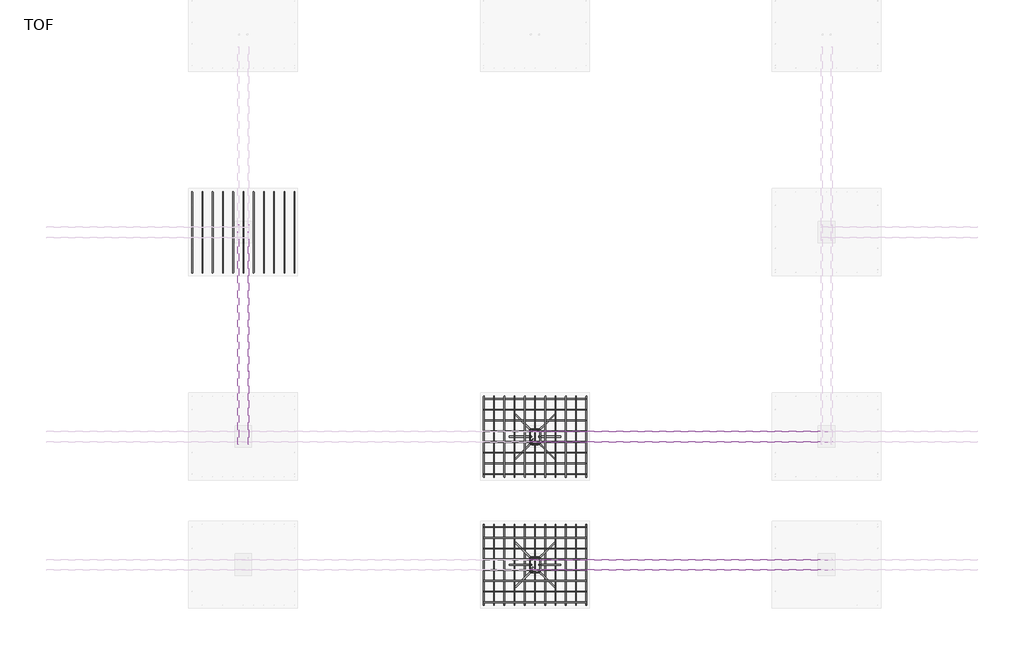
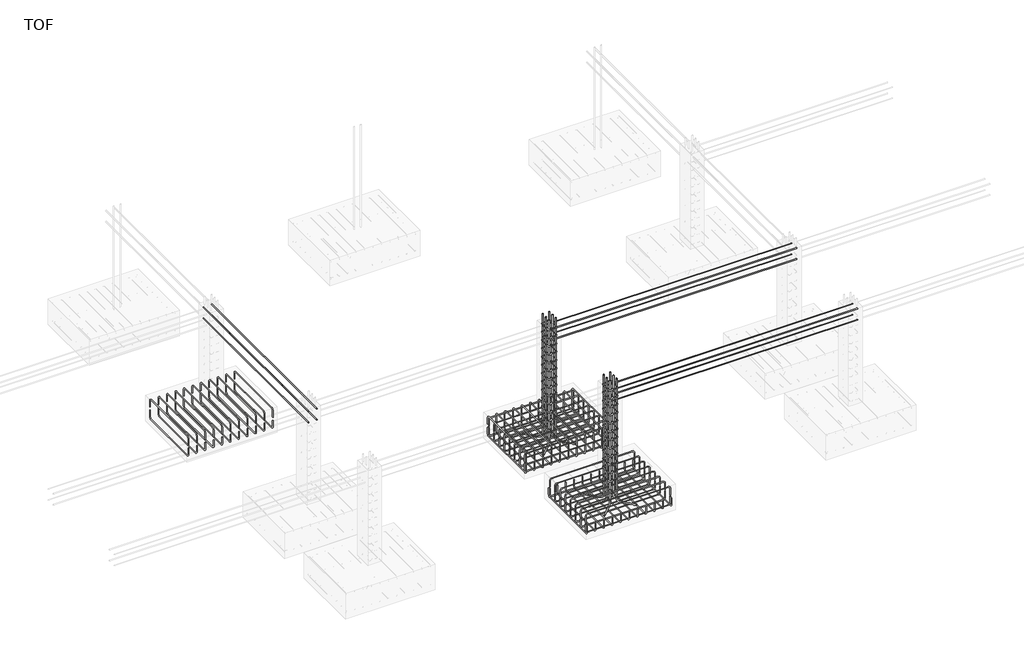
# One storey, part 5 of 10: 35 reinforcing bars.
"""IFC4 building model written with IfcOpenShell, lengths in millimetres."""

from ifc_helpers import new_model, si_unit, point, frame, origin, place, context, project, spatial, polyline, circle_curve, trimmed, segment, composite_curve, source, transform, mapped, element, save
from ifc_brep_helpers import swept_disk

model = new_model("IFC4")

# Units and contexts
model_context = context("Model", 3, world=origin())
ifc_project = project(units=[si_unit("LENGTHUNIT", "METRE", prefix="MILLI")], contexts=[model_context])

# Site, building, storey
site = spatial("IfcSite", under=ifc_project)
building = spatial("IfcBuilding", under=site)
storey = spatial("IfcBuildingStorey", under=building, Name="TOF", Elevation=-1828.8)

# Reinforcing bars
placement = place(None, origin())
reinforcing_bar_shape = source(origin(), model_context, "Body", "SolidModel", [
    swept_disk(composite_curve([segment(polyline([(6330.2782143, -15649.6267376, -2077.5233378), (6330.2782143, -15649.6267376, -2187.5233378)]), True, "CONTINUOUS"), segment(trimmed(circle_curve(frame((6330.2782143, -15614.6267376, -2187.5233378), z_axis=(1.0, 0.0, 0.0), x_axis=(0.0, -35.0, 0.0)), 35.0), [point((6330.2782143, -15649.6267376, -2187.5233378))], [point((6330.2782143, -15614.6267376, -2222.5233378))], True, "CARTESIAN"), True, "CONTINUOUS"), segment(polyline([(6330.2782143, -15614.6267376, -2222.5233378), (6330.2782143, -14574.6267376, -2222.5233378)]), True, "CONTINUOUS"), segment(trimmed(circle_curve(frame((6330.2782143, -14574.6267376, -2187.5233378), z_axis=(1.0, 0.0, 0.0), x_axis=(0.0, 0.0, -35.0)), 35.0), [point((6330.2782143, -14574.6267376, -2222.5233378))], [point((6330.2782143, -14539.6267376, -2187.5233378))], True, "CARTESIAN"), True, "CONTINUOUS"), segment(polyline([(6330.2782143, -14539.6267376, -2187.5233378), (6330.2782143, -14539.6267376, -2077.5233378)]), True, "CONTINUOUS")], self_intersect=False), 5.0),
])
element("IfcReinforcingBar", 1, at=placement, inside=storey, context=model_context, shape_type="MappedRepresentation", body=[
    mapped(reinforcing_bar_shape, transform((0.0, 0.0, 0.0), x_axis=(1.0, 0.0, 0.0), y_axis=(0.0, 1.0, 0.0), z_axis=(0.0, 0.0, 1.0))),
    mapped(reinforcing_bar_shape, transform((-141.0, 0.0, 0.0), x_axis=(1.0, 0.0, 0.0), y_axis=(0.0, 1.0, 0.0), z_axis=(0.0, 0.0, 1.0))),
    mapped(reinforcing_bar_shape, transform((-282.0, 0.0, 0.0), x_axis=(1.0, 0.0, 0.0), y_axis=(0.0, 1.0, 0.0), z_axis=(0.0, 0.0, 1.0))),
    mapped(reinforcing_bar_shape, transform((-423.0, 0.0, 0.0), x_axis=(1.0, 0.0, 0.0), y_axis=(0.0, 1.0, 0.0), z_axis=(0.0, 0.0, 1.0))),
    mapped(reinforcing_bar_shape, transform((-564.0, 0.0, 0.0), x_axis=(1.0, 0.0, 0.0), y_axis=(0.0, 1.0, 0.0), z_axis=(0.0, 0.0, 1.0))),
    mapped(reinforcing_bar_shape, transform((-705.0, 0.0, 0.0), x_axis=(1.0, 0.0, 0.0), y_axis=(0.0, 1.0, 0.0), z_axis=(0.0, 0.0, 1.0))),
    mapped(reinforcing_bar_shape, transform((-846.0, 0.0, 0.0), x_axis=(1.0, 0.0, 0.0), y_axis=(0.0, 1.0, 0.0), z_axis=(0.0, 0.0, 1.0))),
    mapped(reinforcing_bar_shape, transform((-987.0, 0.0, 0.0), x_axis=(1.0, 0.0, 0.0), y_axis=(0.0, 1.0, 0.0), z_axis=(0.0, 0.0, 1.0))),
    mapped(reinforcing_bar_shape, transform((-1128.0, 0.0, 0.0), x_axis=(1.0, 0.0, 0.0), y_axis=(0.0, 1.0, 0.0), z_axis=(0.0, 0.0, 1.0))),
    mapped(reinforcing_bar_shape, transform((-1269.0, 0.0, 0.0), x_axis=(1.0, 0.0, 0.0), y_axis=(0.0, 1.0, 0.0), z_axis=(0.0, 0.0, 1.0))),
    mapped(reinforcing_bar_shape, transform((-1410.0, 0.0, 0.0), x_axis=(1.0, 0.0, 0.0), y_axis=(0.0, 1.0, 0.0), z_axis=(0.0, 0.0, 1.0))),
])
reinforcing_bar_2_shape = source(origin(), model_context, "Body", "SolidModel", [
    swept_disk(composite_curve([segment(polyline([(6330.2782143, -14574.6861459, -2066.1776706), (6330.2782143, -14574.6861459, -2176.1776706)]), True, "CONTINUOUS"), segment(trimmed(circle_curve(frame((6295.2782143, -14574.6861459, -2176.1776706), z_axis=(0.0, 1.0, 0.0), x_axis=(35.0, 0.0, 0.0)), 35.0), [point((6330.2782143, -14574.6861459, -2176.1776706))], [point((6295.2782143, -14574.6861459, -2211.1776706))], True, "CARTESIAN"), True, "CONTINUOUS"), segment(polyline([(6295.2782143, -14574.6861459, -2211.1776706), (4955.2782143, -14574.6861459, -2211.1776706)]), True, "CONTINUOUS"), segment(trimmed(circle_curve(frame((4955.2782143, -14574.6861459, -2176.1776706), z_axis=(0.0, 1.0, 0.0), x_axis=(0.0, 0.0, -35.0)), 35.0), [point((4955.2782143, -14574.6861459, -2211.1776706))], [point((4920.2782143, -14574.6861459, -2176.1776706))], True, "CARTESIAN"), True, "CONTINUOUS"), segment(polyline([(4920.2782143, -14574.6861459, -2176.1776706), (4920.2782143, -14574.6861459, -2066.1776706)]), True, "CONTINUOUS")], self_intersect=False), 5.0),
])
element("IfcReinforcingBar", 2, at=placement, inside=storey, context=model_context, shape_type="MappedRepresentation", body=[
    mapped(reinforcing_bar_2_shape, transform((0.0, 0.0, 0.0), x_axis=(1.0, 0.0, 0.0), y_axis=(0.0, 1.0, 0.0), z_axis=(0.0, 0.0, 1.0))),
    mapped(reinforcing_bar_2_shape, transform((0.0, -148.0321606, 0.0), x_axis=(1.0, 0.0, 0.0), y_axis=(0.0, 1.0, 0.0), z_axis=(0.0, 0.0, 1.0))),
    mapped(reinforcing_bar_2_shape, transform((0.0, -296.0643211, 0.0), x_axis=(1.0, 0.0, 0.0), y_axis=(0.0, 1.0, 0.0), z_axis=(0.0, 0.0, 1.0))),
    mapped(reinforcing_bar_2_shape, transform((0.0, -444.0964817, 0.0), x_axis=(1.0, 0.0, 0.0), y_axis=(0.0, 1.0, 0.0), z_axis=(0.0, 0.0, 1.0))),
    mapped(reinforcing_bar_2_shape, transform((0.0, -592.1286423, 0.0), x_axis=(1.0, 0.0, 0.0), y_axis=(0.0, 1.0, 0.0), z_axis=(0.0, 0.0, 1.0))),
    mapped(reinforcing_bar_2_shape, transform((0.0, -740.1608029, 0.0), x_axis=(1.0, 0.0, 0.0), y_axis=(0.0, 1.0, 0.0), z_axis=(0.0, 0.0, 1.0))),
    mapped(reinforcing_bar_2_shape, transform((0.0, -888.1929634, 0.0), x_axis=(1.0, 0.0, 0.0), y_axis=(0.0, 1.0, 0.0), z_axis=(0.0, 0.0, 1.0))),
    mapped(reinforcing_bar_2_shape, transform((0.0, -1036.225124, 0.0), x_axis=(1.0, 0.0, 0.0), y_axis=(0.0, 1.0, 0.0), z_axis=(0.0, 0.0, 1.0))),
])
reinforcing_bar_3_shape = source(origin(), model_context, "Body", "SolidModel", [
    swept_disk(composite_curve([segment(polyline([(6330.2782143, -15610.9112699, -2039.256778), (6330.2782143, -15610.9112699, -1929.256778)]), True, "CONTINUOUS"), segment(trimmed(circle_curve(frame((6295.2782143, -15610.9112699, -1929.256778), z_axis=(0.0, -1.0, 0.0), x_axis=(35.0, 0.0, 0.0)), 35.0), [point((6330.2782143, -15610.9112699, -1929.256778))], [point((6295.2782143, -15610.9112699, -1894.256778))], True, "CARTESIAN"), True, "CONTINUOUS"), segment(polyline([(6295.2782143, -15610.9112699, -1894.256778), (4955.2782143, -15610.9112699, -1894.256778)]), True, "CONTINUOUS"), segment(trimmed(circle_curve(frame((4955.2782143, -15610.9112699, -1929.256778), z_axis=(0.0, -1.0, 0.0), x_axis=(0.0, 0.0, 35.0)), 35.0), [point((4955.2782143, -15610.9112699, -1894.256778))], [point((4920.2782143, -15610.9112699, -1929.256778))], True, "CARTESIAN"), True, "CONTINUOUS"), segment(polyline([(4920.2782143, -15610.9112699, -1929.256778), (4920.2782143, -15610.9112699, -2039.256778)]), True, "CONTINUOUS")], self_intersect=False), 5.0),
])
element("IfcReinforcingBar", 3, at=placement, inside=storey, context=model_context, shape_type="MappedRepresentation", body=[
    mapped(reinforcing_bar_3_shape, transform((0.0, 0.0, 0.0), x_axis=(1.0, 0.0, 0.0), y_axis=(0.0, 1.0, 0.0), z_axis=(0.0, 0.0, 1.0))),
    mapped(reinforcing_bar_3_shape, transform((0.0, 148.0321606, 0.0), x_axis=(1.0, 0.0, 0.0), y_axis=(0.0, 1.0, 0.0), z_axis=(0.0, 0.0, 1.0))),
    mapped(reinforcing_bar_3_shape, transform((0.0, 296.0643211, 0.0), x_axis=(1.0, 0.0, 0.0), y_axis=(0.0, 1.0, 0.0), z_axis=(0.0, 0.0, 1.0))),
    mapped(reinforcing_bar_3_shape, transform((0.0, 444.0964817, 0.0), x_axis=(1.0, 0.0, 0.0), y_axis=(0.0, 1.0, 0.0), z_axis=(0.0, 0.0, 1.0))),
    mapped(reinforcing_bar_3_shape, transform((0.0, 592.1286423, 0.0), x_axis=(1.0, 0.0, 0.0), y_axis=(0.0, 1.0, 0.0), z_axis=(0.0, 0.0, 1.0))),
    mapped(reinforcing_bar_3_shape, transform((0.0, 740.1608029, 0.0), x_axis=(1.0, 0.0, 0.0), y_axis=(0.0, 1.0, 0.0), z_axis=(0.0, 0.0, 1.0))),
    mapped(reinforcing_bar_3_shape, transform((0.0, 888.1929634, 0.0), x_axis=(1.0, 0.0, 0.0), y_axis=(0.0, 1.0, 0.0), z_axis=(0.0, 0.0, 1.0))),
    mapped(reinforcing_bar_3_shape, transform((0.0, 1036.225124, 0.0), x_axis=(1.0, 0.0, 0.0), y_axis=(0.0, 1.0, 0.0), z_axis=(0.0, 0.0, 1.0))),
])
reinforcing_bar_4_shape = source(origin(), model_context, "Body", "SolidModel", [
    swept_disk(composite_curve([segment(polyline([(6330.2782143, -12774.6267376, -2018.8), (6330.2782143, -12774.6267376, -1908.8)]), True, "CONTINUOUS"), segment(trimmed(circle_curve(frame((6330.2782143, -12809.6267376, -1908.8), z_axis=(1.0, 0.0, 0.0), x_axis=(0.0, 35.0, 0.0)), 35.0), [point((6330.2782143, -12774.6267376, -1908.8))], [point((6330.2782143, -12809.6267376, -1873.8))], True, "CARTESIAN"), True, "CONTINUOUS"), segment(polyline([(6330.2782143, -12809.6267376, -1873.8), (6330.2782143, -13849.6267376, -1873.8)]), True, "CONTINUOUS"), segment(trimmed(circle_curve(frame((6330.2782143, -13849.6267376, -1908.8), z_axis=(1.0, 0.0, 0.0), x_axis=(0.0, 0.0, 35.0)), 35.0), [point((6330.2782143, -13849.6267376, -1873.8))], [point((6330.2782143, -13884.6267376, -1908.8))], True, "CARTESIAN"), True, "CONTINUOUS"), segment(polyline([(6330.2782143, -13884.6267376, -1908.8), (6330.2782143, -13884.6267376, -2018.8)]), True, "CONTINUOUS")], self_intersect=False), 5.0),
])
element("IfcReinforcingBar", 4, at=placement, inside=storey, context=model_context, shape_type="MappedRepresentation", body=[
    mapped(reinforcing_bar_4_shape, transform((0.0, 0.0, 0.0), x_axis=(1.0, 0.0, 0.0), y_axis=(0.0, 1.0, 0.0), z_axis=(0.0, 0.0, 1.0))),
    mapped(reinforcing_bar_4_shape, transform((-141.0, 0.0, 0.0), x_axis=(1.0, 0.0, 0.0), y_axis=(0.0, 1.0, 0.0), z_axis=(0.0, 0.0, 1.0))),
    mapped(reinforcing_bar_4_shape, transform((-282.0, 0.0, 0.0), x_axis=(1.0, 0.0, 0.0), y_axis=(0.0, 1.0, 0.0), z_axis=(0.0, 0.0, 1.0))),
    mapped(reinforcing_bar_4_shape, transform((-423.0, 0.0, 0.0), x_axis=(1.0, 0.0, 0.0), y_axis=(0.0, 1.0, 0.0), z_axis=(0.0, 0.0, 1.0))),
    mapped(reinforcing_bar_4_shape, transform((-564.0, 0.0, 0.0), x_axis=(1.0, 0.0, 0.0), y_axis=(0.0, 1.0, 0.0), z_axis=(0.0, 0.0, 1.0))),
    mapped(reinforcing_bar_4_shape, transform((-705.0, 0.0, 0.0), x_axis=(1.0, 0.0, 0.0), y_axis=(0.0, 1.0, 0.0), z_axis=(0.0, 0.0, 1.0))),
    mapped(reinforcing_bar_4_shape, transform((-846.0, 0.0, 0.0), x_axis=(1.0, 0.0, 0.0), y_axis=(0.0, 1.0, 0.0), z_axis=(0.0, 0.0, 1.0))),
    mapped(reinforcing_bar_4_shape, transform((-987.0, 0.0, 0.0), x_axis=(1.0, 0.0, 0.0), y_axis=(0.0, 1.0, 0.0), z_axis=(0.0, 0.0, 1.0))),
    mapped(reinforcing_bar_4_shape, transform((-1128.0, 0.0, 0.0), x_axis=(1.0, 0.0, 0.0), y_axis=(0.0, 1.0, 0.0), z_axis=(0.0, 0.0, 1.0))),
    mapped(reinforcing_bar_4_shape, transform((-1269.0, 0.0, 0.0), x_axis=(1.0, 0.0, 0.0), y_axis=(0.0, 1.0, 0.0), z_axis=(0.0, 0.0, 1.0))),
    mapped(reinforcing_bar_4_shape, transform((-1410.0, 0.0, 0.0), x_axis=(1.0, 0.0, 0.0), y_axis=(0.0, 1.0, 0.0), z_axis=(0.0, 0.0, 1.0))),
])
reinforcing_bar_5_shape = source(origin(), model_context, "Body", "SolidModel", [
    swept_disk(composite_curve([segment(polyline([(6330.2782143, -13884.6267376, -2077.5233378), (6330.2782143, -13884.6267376, -2187.5233378)]), True, "CONTINUOUS"), segment(trimmed(circle_curve(frame((6330.2782143, -13849.6267376, -2187.5233378), z_axis=(1.0, 0.0, 0.0), x_axis=(0.0, -35.0, 0.0)), 35.0), [point((6330.2782143, -13884.6267376, -2187.5233378))], [point((6330.2782143, -13849.6267376, -2222.5233378))], True, "CARTESIAN"), True, "CONTINUOUS"), segment(polyline([(6330.2782143, -13849.6267376, -2222.5233378), (6330.2782143, -12809.6267376, -2222.5233378)]), True, "CONTINUOUS"), segment(trimmed(circle_curve(frame((6330.2782143, -12809.6267376, -2187.5233378), z_axis=(1.0, 0.0, 0.0), x_axis=(0.0, 0.0, -35.0)), 35.0), [point((6330.2782143, -12809.6267376, -2222.5233378))], [point((6330.2782143, -12774.6267376, -2187.5233378))], True, "CARTESIAN"), True, "CONTINUOUS"), segment(polyline([(6330.2782143, -12774.6267376, -2187.5233378), (6330.2782143, -12774.6267376, -2077.5233378)]), True, "CONTINUOUS")], self_intersect=False), 5.0),
])
element("IfcReinforcingBar", 5, at=placement, inside=storey, context=model_context, shape_type="MappedRepresentation", body=[
    mapped(reinforcing_bar_5_shape, transform((0.0, 0.0, 0.0), x_axis=(1.0, 0.0, 0.0), y_axis=(0.0, 1.0, 0.0), z_axis=(0.0, 0.0, 1.0))),
    mapped(reinforcing_bar_5_shape, transform((-141.0, 0.0, 0.0), x_axis=(1.0, 0.0, 0.0), y_axis=(0.0, 1.0, 0.0), z_axis=(0.0, 0.0, 1.0))),
    mapped(reinforcing_bar_5_shape, transform((-282.0, 0.0, 0.0), x_axis=(1.0, 0.0, 0.0), y_axis=(0.0, 1.0, 0.0), z_axis=(0.0, 0.0, 1.0))),
    mapped(reinforcing_bar_5_shape, transform((-423.0, 0.0, 0.0), x_axis=(1.0, 0.0, 0.0), y_axis=(0.0, 1.0, 0.0), z_axis=(0.0, 0.0, 1.0))),
    mapped(reinforcing_bar_5_shape, transform((-564.0, 0.0, 0.0), x_axis=(1.0, 0.0, 0.0), y_axis=(0.0, 1.0, 0.0), z_axis=(0.0, 0.0, 1.0))),
    mapped(reinforcing_bar_5_shape, transform((-705.0, 0.0, 0.0), x_axis=(1.0, 0.0, 0.0), y_axis=(0.0, 1.0, 0.0), z_axis=(0.0, 0.0, 1.0))),
    mapped(reinforcing_bar_5_shape, transform((-846.0, 0.0, 0.0), x_axis=(1.0, 0.0, 0.0), y_axis=(0.0, 1.0, 0.0), z_axis=(0.0, 0.0, 1.0))),
    mapped(reinforcing_bar_5_shape, transform((-987.0, 0.0, 0.0), x_axis=(1.0, 0.0, 0.0), y_axis=(0.0, 1.0, 0.0), z_axis=(0.0, 0.0, 1.0))),
    mapped(reinforcing_bar_5_shape, transform((-1128.0, 0.0, 0.0), x_axis=(1.0, 0.0, 0.0), y_axis=(0.0, 1.0, 0.0), z_axis=(0.0, 0.0, 1.0))),
    mapped(reinforcing_bar_5_shape, transform((-1269.0, 0.0, 0.0), x_axis=(1.0, 0.0, 0.0), y_axis=(0.0, 1.0, 0.0), z_axis=(0.0, 0.0, 1.0))),
    mapped(reinforcing_bar_5_shape, transform((-1410.0, 0.0, 0.0), x_axis=(1.0, 0.0, 0.0), y_axis=(0.0, 1.0, 0.0), z_axis=(0.0, 0.0, 1.0))),
])
reinforcing_bar_6_shape = source(origin(), model_context, "Body", "SolidModel", [
    swept_disk(composite_curve([segment(polyline([(6330.2782143, -12809.6861459, -2066.1776706), (6330.2782143, -12809.6861459, -2176.1776706)]), True, "CONTINUOUS"), segment(trimmed(circle_curve(frame((6295.2782143, -12809.6861459, -2176.1776706), z_axis=(0.0, 1.0, 0.0), x_axis=(35.0, 0.0, 0.0)), 35.0), [point((6330.2782143, -12809.6861459, -2176.1776706))], [point((6295.2782143, -12809.6861459, -2211.1776706))], True, "CARTESIAN"), True, "CONTINUOUS"), segment(polyline([(6295.2782143, -12809.6861459, -2211.1776706), (4955.2782143, -12809.6861459, -2211.1776706)]), True, "CONTINUOUS"), segment(trimmed(circle_curve(frame((4955.2782143, -12809.6861459, -2176.1776706), z_axis=(0.0, 1.0, 0.0), x_axis=(0.0, 0.0, -35.0)), 35.0), [point((4955.2782143, -12809.6861459, -2211.1776706))], [point((4920.2782143, -12809.6861459, -2176.1776706))], True, "CARTESIAN"), True, "CONTINUOUS"), segment(polyline([(4920.2782143, -12809.6861459, -2176.1776706), (4920.2782143, -12809.6861459, -2066.1776706)]), True, "CONTINUOUS")], self_intersect=False), 5.0),
])
element("IfcReinforcingBar", 6, at=placement, inside=storey, context=model_context, shape_type="MappedRepresentation", body=[
    mapped(reinforcing_bar_6_shape, transform((0.0, 0.0, 0.0), x_axis=(1.0, 0.0, 0.0), y_axis=(0.0, 1.0, 0.0), z_axis=(0.0, 0.0, 1.0))),
    mapped(reinforcing_bar_6_shape, transform((0.0, -148.0321606, 0.0), x_axis=(1.0, 0.0, 0.0), y_axis=(0.0, 1.0, 0.0), z_axis=(0.0, 0.0, 1.0))),
    mapped(reinforcing_bar_6_shape, transform((0.0, -296.0643211, 0.0), x_axis=(1.0, 0.0, 0.0), y_axis=(0.0, 1.0, 0.0), z_axis=(0.0, 0.0, 1.0))),
    mapped(reinforcing_bar_6_shape, transform((0.0, -444.0964817, 0.0), x_axis=(1.0, 0.0, 0.0), y_axis=(0.0, 1.0, 0.0), z_axis=(0.0, 0.0, 1.0))),
    mapped(reinforcing_bar_6_shape, transform((0.0, -592.1286423, 0.0), x_axis=(1.0, 0.0, 0.0), y_axis=(0.0, 1.0, 0.0), z_axis=(0.0, 0.0, 1.0))),
    mapped(reinforcing_bar_6_shape, transform((0.0, -740.1608029, 0.0), x_axis=(1.0, 0.0, 0.0), y_axis=(0.0, 1.0, 0.0), z_axis=(0.0, 0.0, 1.0))),
    mapped(reinforcing_bar_6_shape, transform((0.0, -888.1929634, 0.0), x_axis=(1.0, 0.0, 0.0), y_axis=(0.0, 1.0, 0.0), z_axis=(0.0, 0.0, 1.0))),
    mapped(reinforcing_bar_6_shape, transform((0.0, -1036.225124, 0.0), x_axis=(1.0, 0.0, 0.0), y_axis=(0.0, 1.0, 0.0), z_axis=(0.0, 0.0, 1.0))),
])
reinforcing_bar_7_shape = source(origin(), model_context, "Body", "SolidModel", [
    swept_disk(composite_curve([segment(polyline([(6330.2782143, -13845.9112699, -2039.256778), (6330.2782143, -13845.9112699, -1929.256778)]), True, "CONTINUOUS"), segment(trimmed(circle_curve(frame((6295.2782143, -13845.9112699, -1929.256778), z_axis=(0.0, -1.0, 0.0), x_axis=(35.0, 0.0, 0.0)), 35.0), [point((6330.2782143, -13845.9112699, -1929.256778))], [point((6295.2782143, -13845.9112699, -1894.256778))], True, "CARTESIAN"), True, "CONTINUOUS"), segment(polyline([(6295.2782143, -13845.9112699, -1894.256778), (4955.2782143, -13845.9112699, -1894.256778)]), True, "CONTINUOUS"), segment(trimmed(circle_curve(frame((4955.2782143, -13845.9112699, -1929.256778), z_axis=(0.0, -1.0, 0.0), x_axis=(0.0, 0.0, 35.0)), 35.0), [point((4955.2782143, -13845.9112699, -1894.256778))], [point((4920.2782143, -13845.9112699, -1929.256778))], True, "CARTESIAN"), True, "CONTINUOUS"), segment(polyline([(4920.2782143, -13845.9112699, -1929.256778), (4920.2782143, -13845.9112699, -2039.256778)]), True, "CONTINUOUS")], self_intersect=False), 5.0),
])
element("IfcReinforcingBar", 7, at=placement, inside=storey, context=model_context, shape_type="MappedRepresentation", body=[
    mapped(reinforcing_bar_7_shape, transform((0.0, 0.0, 0.0), x_axis=(1.0, 0.0, 0.0), y_axis=(0.0, 1.0, 0.0), z_axis=(0.0, 0.0, 1.0))),
    mapped(reinforcing_bar_7_shape, transform((0.0, 148.0321606, 0.0), x_axis=(1.0, 0.0, 0.0), y_axis=(0.0, 1.0, 0.0), z_axis=(0.0, 0.0, 1.0))),
    mapped(reinforcing_bar_7_shape, transform((0.0, 296.0643211, 0.0), x_axis=(1.0, 0.0, 0.0), y_axis=(0.0, 1.0, 0.0), z_axis=(0.0, 0.0, 1.0))),
    mapped(reinforcing_bar_7_shape, transform((0.0, 444.0964817, 0.0), x_axis=(1.0, 0.0, 0.0), y_axis=(0.0, 1.0, 0.0), z_axis=(0.0, 0.0, 1.0))),
    mapped(reinforcing_bar_7_shape, transform((0.0, 592.1286423, 0.0), x_axis=(1.0, 0.0, 0.0), y_axis=(0.0, 1.0, 0.0), z_axis=(0.0, 0.0, 1.0))),
    mapped(reinforcing_bar_7_shape, transform((0.0, 740.1608029, 0.0), x_axis=(1.0, 0.0, 0.0), y_axis=(0.0, 1.0, 0.0), z_axis=(0.0, 0.0, 1.0))),
    mapped(reinforcing_bar_7_shape, transform((0.0, 888.1929634, 0.0), x_axis=(1.0, 0.0, 0.0), y_axis=(0.0, 1.0, 0.0), z_axis=(0.0, 0.0, 1.0))),
    mapped(reinforcing_bar_7_shape, transform((0.0, 1036.225124, 0.0), x_axis=(1.0, 0.0, 0.0), y_axis=(0.0, 1.0, 0.0), z_axis=(0.0, 0.0, 1.0))),
])
reinforcing_bar_8_shape = source(origin(), model_context, "Body", "SolidModel", [
    swept_disk(composite_curve([segment(polyline([(2315.2782143, -9959.6267376, -2018.8), (2315.2782143, -9959.6267376, -1908.8)]), True, "CONTINUOUS"), segment(trimmed(circle_curve(frame((2315.2782143, -9994.6267376, -1908.8), z_axis=(1.0, 0.0, 0.0), x_axis=(0.0, 35.0, 0.0)), 35.0), [point((2315.2782143, -9959.6267376, -1908.8))], [point((2315.2782143, -9994.6267376, -1873.8))], True, "CARTESIAN"), True, "CONTINUOUS"), segment(polyline([(2315.2782143, -9994.6267376, -1873.8), (2315.2782143, -11034.6267376, -1873.8)]), True, "CONTINUOUS"), segment(trimmed(circle_curve(frame((2315.2782143, -11034.6267376, -1908.8), z_axis=(1.0, 0.0, 0.0), x_axis=(0.0, 0.0, 35.0)), 35.0), [point((2315.2782143, -11034.6267376, -1873.8))], [point((2315.2782143, -11069.6267376, -1908.8))], True, "CARTESIAN"), True, "CONTINUOUS"), segment(polyline([(2315.2782143, -11069.6267376, -1908.8), (2315.2782143, -11069.6267376, -2018.8)]), True, "CONTINUOUS")], self_intersect=False), 5.0),
])
element("IfcReinforcingBar", 8, at=placement, inside=storey, context=model_context, shape_type="MappedRepresentation", body=[
    mapped(reinforcing_bar_8_shape, transform((0.0, 0.0, 0.0), x_axis=(1.0, 0.0, 0.0), y_axis=(0.0, 1.0, 0.0), z_axis=(0.0, 0.0, 1.0))),
    mapped(reinforcing_bar_8_shape, transform((-141.0, 0.0, 0.0), x_axis=(1.0, 0.0, 0.0), y_axis=(0.0, 1.0, 0.0), z_axis=(0.0, 0.0, 1.0))),
    mapped(reinforcing_bar_8_shape, transform((-282.0, 0.0, 0.0), x_axis=(1.0, 0.0, 0.0), y_axis=(0.0, 1.0, 0.0), z_axis=(0.0, 0.0, 1.0))),
    mapped(reinforcing_bar_8_shape, transform((-423.0, 0.0, 0.0), x_axis=(1.0, 0.0, 0.0), y_axis=(0.0, 1.0, 0.0), z_axis=(0.0, 0.0, 1.0))),
    mapped(reinforcing_bar_8_shape, transform((-564.0, 0.0, 0.0), x_axis=(1.0, 0.0, 0.0), y_axis=(0.0, 1.0, 0.0), z_axis=(0.0, 0.0, 1.0))),
    mapped(reinforcing_bar_8_shape, transform((-705.0, 0.0, 0.0), x_axis=(1.0, 0.0, 0.0), y_axis=(0.0, 1.0, 0.0), z_axis=(0.0, 0.0, 1.0))),
    mapped(reinforcing_bar_8_shape, transform((-846.0, 0.0, 0.0), x_axis=(1.0, 0.0, 0.0), y_axis=(0.0, 1.0, 0.0), z_axis=(0.0, 0.0, 1.0))),
    mapped(reinforcing_bar_8_shape, transform((-987.0, 0.0, 0.0), x_axis=(1.0, 0.0, 0.0), y_axis=(0.0, 1.0, 0.0), z_axis=(0.0, 0.0, 1.0))),
    mapped(reinforcing_bar_8_shape, transform((-1128.0, 0.0, 0.0), x_axis=(1.0, 0.0, 0.0), y_axis=(0.0, 1.0, 0.0), z_axis=(0.0, 0.0, 1.0))),
    mapped(reinforcing_bar_8_shape, transform((-1269.0, 0.0, 0.0), x_axis=(1.0, 0.0, 0.0), y_axis=(0.0, 1.0, 0.0), z_axis=(0.0, 0.0, 1.0))),
    mapped(reinforcing_bar_8_shape, transform((-1410.0, 0.0, 0.0), x_axis=(1.0, 0.0, 0.0), y_axis=(0.0, 1.0, 0.0), z_axis=(0.0, 0.0, 1.0))),
])
reinforcing_bar_9_shape = source(origin(), model_context, "Body", "SolidModel", [
    swept_disk(composite_curve([segment(polyline([(2315.2782143, -11069.6267376, -2077.5233378), (2315.2782143, -11069.6267376, -2187.5233378)]), True, "CONTINUOUS"), segment(trimmed(circle_curve(frame((2315.2782143, -11034.6267376, -2187.5233378), z_axis=(1.0, 0.0, 0.0), x_axis=(0.0, -35.0, 0.0)), 35.0), [point((2315.2782143, -11069.6267376, -2187.5233378))], [point((2315.2782143, -11034.6267376, -2222.5233378))], True, "CARTESIAN"), True, "CONTINUOUS"), segment(polyline([(2315.2782143, -11034.6267376, -2222.5233378), (2315.2782143, -9994.6267376, -2222.5233378)]), True, "CONTINUOUS"), segment(trimmed(circle_curve(frame((2315.2782143, -9994.6267376, -2187.5233378), z_axis=(1.0, 0.0, 0.0), x_axis=(0.0, 0.0, -35.0)), 35.0), [point((2315.2782143, -9994.6267376, -2222.5233378))], [point((2315.2782143, -9959.6267376, -2187.5233378))], True, "CARTESIAN"), True, "CONTINUOUS"), segment(polyline([(2315.2782143, -9959.6267376, -2187.5233378), (2315.2782143, -9959.6267376, -2077.5233378)]), True, "CONTINUOUS")], self_intersect=False), 5.0),
])
element("IfcReinforcingBar", 9, at=placement, inside=storey, context=model_context, shape_type="MappedRepresentation", body=[
    mapped(reinforcing_bar_9_shape, transform((0.0, 0.0, 0.0), x_axis=(1.0, 0.0, 0.0), y_axis=(0.0, 1.0, 0.0), z_axis=(0.0, 0.0, 1.0))),
    mapped(reinforcing_bar_9_shape, transform((-141.0, 0.0, 0.0), x_axis=(1.0, 0.0, 0.0), y_axis=(0.0, 1.0, 0.0), z_axis=(0.0, 0.0, 1.0))),
    mapped(reinforcing_bar_9_shape, transform((-282.0, 0.0, 0.0), x_axis=(1.0, 0.0, 0.0), y_axis=(0.0, 1.0, 0.0), z_axis=(0.0, 0.0, 1.0))),
    mapped(reinforcing_bar_9_shape, transform((-423.0, 0.0, 0.0), x_axis=(1.0, 0.0, 0.0), y_axis=(0.0, 1.0, 0.0), z_axis=(0.0, 0.0, 1.0))),
    mapped(reinforcing_bar_9_shape, transform((-564.0, 0.0, 0.0), x_axis=(1.0, 0.0, 0.0), y_axis=(0.0, 1.0, 0.0), z_axis=(0.0, 0.0, 1.0))),
    mapped(reinforcing_bar_9_shape, transform((-705.0, 0.0, 0.0), x_axis=(1.0, 0.0, 0.0), y_axis=(0.0, 1.0, 0.0), z_axis=(0.0, 0.0, 1.0))),
    mapped(reinforcing_bar_9_shape, transform((-846.0, 0.0, 0.0), x_axis=(1.0, 0.0, 0.0), y_axis=(0.0, 1.0, 0.0), z_axis=(0.0, 0.0, 1.0))),
    mapped(reinforcing_bar_9_shape, transform((-987.0, 0.0, 0.0), x_axis=(1.0, 0.0, 0.0), y_axis=(0.0, 1.0, 0.0), z_axis=(0.0, 0.0, 1.0))),
    mapped(reinforcing_bar_9_shape, transform((-1128.0, 0.0, 0.0), x_axis=(1.0, 0.0, 0.0), y_axis=(0.0, 1.0, 0.0), z_axis=(0.0, 0.0, 1.0))),
    mapped(reinforcing_bar_9_shape, transform((-1269.0, 0.0, 0.0), x_axis=(1.0, 0.0, 0.0), y_axis=(0.0, 1.0, 0.0), z_axis=(0.0, 0.0, 1.0))),
    mapped(reinforcing_bar_9_shape, transform((-1410.0, 0.0, 0.0), x_axis=(1.0, 0.0, 0.0), y_axis=(0.0, 1.0, 0.0), z_axis=(0.0, 0.0, 1.0))),
])
reinforcing_bar_10_shape = source(origin(), model_context, "Body", "SolidModel", [
    swept_disk(composite_curve([segment(polyline([(5595.248777, -15125.7150493, -1784.8), (5561.3076515, -15159.6561748, -1784.8)]), True, "CONTINUOUS"), segment(trimmed(circle_curve(frame((5578.2782143, -15176.6267376, -1784.8), z_axis=(0.0, 0.0, 1.0), x_axis=(-16.970562800000152, 16.970562799999243, 0.0)), 24.0), [point((5561.3076515, -15159.6561748, -1784.8))], [point((5578.2782143, -15200.6267376, -1784.8))], True, "CARTESIAN"), True, "CONTINUOUS"), segment(polyline([(5578.2782143, -15200.6267376, -1784.8), (5672.2782143, -15200.6267376, -1784.8)]), True, "CONTINUOUS"), segment(trimmed(circle_curve(frame((5672.2782143, -15176.6267376, -1784.8), z_axis=(0.0, 0.0, 1.0), x_axis=(0.0, -24.0, 0.0)), 24.0), [point((5672.2782143, -15200.6267376, -1784.8))], [point((5696.2782143, -15176.6267376, -1784.8))], True, "CARTESIAN"), True, "CONTINUOUS"), segment(polyline([(5696.2782143, -15176.6267376, -1784.8), (5696.2782143, -15012.6267376, -1784.8)]), True, "CONTINUOUS"), segment(trimmed(circle_curve(frame((5672.3162115, -15012.6267376, -1786.149972), z_axis=(-0.05624883273897078, 0.0, 0.9984167811167355), x_axis=(23.962002800000846, 0.0, 1.3499719999999797)), 24.0), [point((5696.2782143, -15012.6267376, -1784.8))], [point((5672.3162115, -14988.6267376, -1786.149972))], True, "CARTESIAN"), True, "CONTINUOUS"), segment(polyline([(5672.3162115, -14988.6267376, -1786.149972), (5578.240217, -14988.6267376, -1791.450028)]), True, "CONTINUOUS"), segment(trimmed(circle_curve(frame((5578.240217, -15012.6267376, -1791.450028), z_axis=(-0.05624883273897078, 0.0, 0.9984167811167355), x_axis=(0.0, 24.0, 0.0)), 24.0), [point((5578.240217, -14988.6267376, -1791.450028))], [point((5554.2782143, -15012.6267376, -1792.8))], True, "CARTESIAN"), True, "CONTINUOUS"), segment(polyline([(5554.2782143, -15012.6267376, -1792.8), (5554.2782143, -15176.6267376, -1792.8)]), True, "CONTINUOUS"), segment(trimmed(circle_curve(frame((5578.2782143, -15176.6267376, -1792.8), z_axis=(0.0, 0.0, 1.0), x_axis=(-24.0, 0.0, 0.0)), 24.0), [point((5554.2782143, -15176.6267376, -1792.8))], [point((5595.248777, -15193.5973003, -1792.8))], True, "CARTESIAN"), True, "CONTINUOUS"), segment(polyline([(5595.248777, -15193.5973003, -1792.8), (5629.1899025, -15159.6561748, -1792.8)]), True, "CONTINUOUS")], self_intersect=False), 4.0),
])
element("IfcReinforcingBar", 10, at=placement, inside=storey, context=model_context, shape_type="MappedRepresentation", body=[
    mapped(reinforcing_bar_10_shape, transform((0.0, 0.0, 0.0), x_axis=(1.0, 0.0, 0.0), y_axis=(0.0, 1.0, 0.0), z_axis=(0.0, 0.0, 1.0))),
    mapped(reinforcing_bar_10_shape, transform((0.0, 0.0, 145.9395608), x_axis=(1.0, 0.0, 0.0), y_axis=(0.0, 1.0, 0.0), z_axis=(0.0, 0.0, 1.0))),
    mapped(reinforcing_bar_10_shape, transform((0.0, 0.0, 291.8791216), x_axis=(1.0, 0.0, 0.0), y_axis=(0.0, 1.0, 0.0), z_axis=(0.0, 0.0, 1.0))),
    mapped(reinforcing_bar_10_shape, transform((0.0, 0.0, 437.8186825), x_axis=(1.0, 0.0, 0.0), y_axis=(0.0, 1.0, 0.0), z_axis=(0.0, 0.0, 1.0))),
    mapped(reinforcing_bar_10_shape, transform((0.0, 0.0, 583.7582433), x_axis=(1.0, 0.0, 0.0), y_axis=(0.0, 1.0, 0.0), z_axis=(0.0, 0.0, 1.0))),
    mapped(reinforcing_bar_10_shape, transform((0.0, 0.0, 729.6978041), x_axis=(1.0, 0.0, 0.0), y_axis=(0.0, 1.0, 0.0), z_axis=(0.0, 0.0, 1.0))),
    mapped(reinforcing_bar_10_shape, transform((0.0, 0.0, 875.6373649), x_axis=(1.0, 0.0, 0.0), y_axis=(0.0, 1.0, 0.0), z_axis=(0.0, 0.0, 1.0))),
    mapped(reinforcing_bar_10_shape, transform((0.0, 0.0, 1021.5769258), x_axis=(1.0, 0.0, 0.0), y_axis=(0.0, 1.0, 0.0), z_axis=(0.0, 0.0, 1.0))),
    mapped(reinforcing_bar_10_shape, transform((0.0, 0.0, 1167.5164866), x_axis=(1.0, 0.0, 0.0), y_axis=(0.0, 1.0, 0.0), z_axis=(0.0, 0.0, 1.0))),
    mapped(reinforcing_bar_10_shape, transform((0.0, 0.0, 1313.4560474), x_axis=(1.0, 0.0, 0.0), y_axis=(0.0, 1.0, 0.0), z_axis=(0.0, 0.0, 1.0))),
    mapped(reinforcing_bar_10_shape, transform((0.0, 0.0, 1459.3956082), x_axis=(1.0, 0.0, 0.0), y_axis=(0.0, 1.0, 0.0), z_axis=(0.0, 0.0, 1.0))),
    mapped(reinforcing_bar_10_shape, transform((0.0, 0.0, 1605.3351691), x_axis=(1.0, 0.0, 0.0), y_axis=(0.0, 1.0, 0.0), z_axis=(0.0, 0.0, 1.0))),
])
element("IfcReinforcingBar", 11, at=placement, inside=storey, context=model_context, shape_type="SolidModel", body=[
    swept_disk(composite_curve([segment(polyline([(5680.884816, -15185.2333393, -20.0), (5680.884816, -15185.2333393, -2138.7824747)]), True, "CONTINUOUS"), segment(trimmed(circle_curve(frame((5720.1292424, -15224.4777657, -2138.7824747), z_axis=(-0.7071067811865545, -0.7071067811865406, 0.0), x_axis=(-39.24442640000052, 39.2444263999987, 0.0)), 55.5), [point((5680.884816, -15185.2333393, -2138.7824747))], [point((5720.1292424, -15224.4777657, -2194.2824747))], True, "CARTESIAN"), True, "CONTINUOUS"), segment(polyline([(5720.1292424, -15224.4777657, -2194.2824747), (5892.5083915, -15396.8569148, -2194.2824747)]), True, "CONTINUOUS")], self_intersect=False), 8.0),
])
element("IfcReinforcingBar", 12, at=placement, inside=storey, context=model_context, shape_type="SolidModel", body=[
    swept_disk(composite_curve([segment(polyline([(5680.934816, -15094.6267376, -20.0), (5680.934816, -15094.6267376, -2138.7824747)]), True, "CONTINUOUS"), segment(trimmed(circle_curve(frame((5736.434816, -15094.6267376, -2138.7824747), z_axis=(0.0, -1.0, 0.0), x_axis=(-55.5, 0.0, 0.0)), 55.5), [point((5680.934816, -15094.6267376, -2138.7824747))], [point((5736.434816, -15094.6267376, -2194.2824747))], True, "CARTESIAN"), True, "CONTINUOUS"), segment(polyline([(5736.434816, -15094.6267376, -2194.2824747), (5980.1657466, -15094.6267376, -2194.2824747)]), True, "CONTINUOUS")], self_intersect=False), 8.0),
])
element("IfcReinforcingBar", 13, at=placement, inside=storey, context=model_context, shape_type="SolidModel", body=[
    swept_disk(composite_curve([segment(polyline([(5680.884816, -15004.0201359, -20.0), (5680.884816, -15004.0201359, -2138.7824747)]), True, "CONTINUOUS"), segment(trimmed(circle_curve(frame((5720.1292424, -14964.7757095, -2138.7824747), z_axis=(0.7071067811865545, -0.7071067811865407, 0.0), x_axis=(-39.24442640000052, -39.24442640000052, 0.0)), 55.5), [point((5680.884816, -15004.0201359, -2138.7824747))], [point((5720.1292424, -14964.7757095, -2194.2824747))], True, "CARTESIAN"), True, "CONTINUOUS"), segment(polyline([(5720.1292424, -14964.7757095, -2194.2824747), (5892.5083915, -14792.3965603, -2194.2824747)]), True, "CONTINUOUS")], self_intersect=False), 8.0),
])
element("IfcReinforcingBar", 14, at=placement, inside=storey, context=model_context, shape_type="SolidModel", body=[
    swept_disk(composite_curve([segment(polyline([(5569.6716126, -15185.2333393, -20.0), (5569.6716126, -15185.2333393, -2138.7824747)]), True, "CONTINUOUS"), segment(trimmed(circle_curve(frame((5530.4271862, -15224.4777657, -2138.7824747), z_axis=(-0.7071067811865517, 0.7071067811865434, 0.0), x_axis=(39.24442640000052, 39.2444263999987, 0.0)), 55.5), [point((5569.6716126, -15185.2333393, -2138.7824747))], [point((5530.4271862, -15224.4777657, -2194.2824747))], True, "CARTESIAN"), True, "CONTINUOUS"), segment(polyline([(5530.4271862, -15224.4777657, -2194.2824747), (5358.048037, -15396.8569148, -2194.2824747)]), True, "CONTINUOUS")], self_intersect=False), 8.0),
])
element("IfcReinforcingBar", 15, at=placement, inside=storey, context=model_context, shape_type="SolidModel", body=[
    swept_disk(composite_curve([segment(polyline([(5569.6216126, -15094.6267376, -20.0), (5569.6216126, -15094.6267376, -2138.7824747)]), True, "CONTINUOUS"), segment(trimmed(circle_curve(frame((5514.1216126, -15094.6267376, -2138.7824747), z_axis=(0.0, 1.0, 0.0), x_axis=(55.5, 0.0, 0.0)), 55.5), [point((5569.6216126, -15094.6267376, -2138.7824747))], [point((5514.1216126, -15094.6267376, -2194.2824747))], True, "CARTESIAN"), True, "CONTINUOUS"), segment(polyline([(5514.1216126, -15094.6267376, -2194.2824747), (5270.3906819, -15094.6267376, -2194.2824747)]), True, "CONTINUOUS")], self_intersect=False), 8.0),
])
element("IfcReinforcingBar", 16, at=placement, inside=storey, context=model_context, shape_type="SolidModel", body=[
    swept_disk(composite_curve([segment(polyline([(5569.6716126, -15004.0201359, -20.0), (5569.6716126, -15004.0201359, -2138.7824747)]), True, "CONTINUOUS"), segment(trimmed(circle_curve(frame((5530.4271862, -14964.7757095, -2138.7824747), z_axis=(0.7071067811865572, 0.7071067811865379, 0.0), x_axis=(39.24442640000052, -39.24442640000052, 0.0)), 55.5), [point((5569.6716126, -15004.0201359, -2138.7824747))], [point((5530.4271862, -14964.7757095, -2194.2824747))], True, "CARTESIAN"), True, "CONTINUOUS"), segment(polyline([(5530.4271862, -14964.7757095, -2194.2824747), (5358.048037, -14792.3965603, -2194.2824747)]), True, "CONTINUOUS")], self_intersect=False), 8.0),
])
reinforcing_bar_11_shape = source(origin(), model_context, "Body", "SolidModel", [
    swept_disk(composite_curve([segment(polyline([(5595.248777, -13360.7150493, -1784.8), (5561.3076515, -13394.6561748, -1784.8)]), True, "CONTINUOUS"), segment(trimmed(circle_curve(frame((5578.2782143, -13411.6267376, -1784.8), z_axis=(0.0, 0.0, 1.0), x_axis=(-16.970562800000152, 16.970562799999243, 0.0)), 24.0), [point((5561.3076515, -13394.6561748, -1784.8))], [point((5578.2782143, -13435.6267376, -1784.8))], True, "CARTESIAN"), True, "CONTINUOUS"), segment(polyline([(5578.2782143, -13435.6267376, -1784.8), (5672.2782143, -13435.6267376, -1784.8)]), True, "CONTINUOUS"), segment(trimmed(circle_curve(frame((5672.2782143, -13411.6267376, -1784.8), z_axis=(0.0, 0.0, 1.0), x_axis=(0.0, -24.0, 0.0)), 24.0), [point((5672.2782143, -13435.6267376, -1784.8))], [point((5696.2782143, -13411.6267376, -1784.8))], True, "CARTESIAN"), True, "CONTINUOUS"), segment(polyline([(5696.2782143, -13411.6267376, -1784.8), (5696.2782143, -13247.6267376, -1784.8)]), True, "CONTINUOUS"), segment(trimmed(circle_curve(frame((5672.3162115, -13247.6267376, -1786.149972), z_axis=(-0.05624883273897078, 0.0, 0.9984167811167355), x_axis=(23.962002800000846, 0.0, 1.3499719999999797)), 24.0), [point((5696.2782143, -13247.6267376, -1784.8))], [point((5672.3162115, -13223.6267376, -1786.149972))], True, "CARTESIAN"), True, "CONTINUOUS"), segment(polyline([(5672.3162115, -13223.6267376, -1786.149972), (5578.240217, -13223.6267376, -1791.450028)]), True, "CONTINUOUS"), segment(trimmed(circle_curve(frame((5578.240217, -13247.6267376, -1791.450028), z_axis=(-0.05624883273897078, 0.0, 0.9984167811167355), x_axis=(0.0, 24.0, 0.0)), 24.0), [point((5578.240217, -13223.6267376, -1791.450028))], [point((5554.2782143, -13247.6267376, -1792.8))], True, "CARTESIAN"), True, "CONTINUOUS"), segment(polyline([(5554.2782143, -13247.6267376, -1792.8), (5554.2782143, -13411.6267376, -1792.8)]), True, "CONTINUOUS"), segment(trimmed(circle_curve(frame((5578.2782143, -13411.6267376, -1792.8), z_axis=(0.0, 0.0, 1.0), x_axis=(-24.0, 0.0, 0.0)), 24.0), [point((5554.2782143, -13411.6267376, -1792.8))], [point((5595.248777, -13428.5973003, -1792.8))], True, "CARTESIAN"), True, "CONTINUOUS"), segment(polyline([(5595.248777, -13428.5973003, -1792.8), (5629.1899025, -13394.6561748, -1792.8)]), True, "CONTINUOUS")], self_intersect=False), 4.0),
])
element("IfcReinforcingBar", 17, at=placement, inside=storey, context=model_context, shape_type="MappedRepresentation", body=[
    mapped(reinforcing_bar_11_shape, transform((0.0, 0.0, 0.0), x_axis=(1.0, 0.0, 0.0), y_axis=(0.0, 1.0, 0.0), z_axis=(0.0, 0.0, 1.0))),
    mapped(reinforcing_bar_11_shape, transform((0.0, 0.0, 145.9395608), x_axis=(1.0, 0.0, 0.0), y_axis=(0.0, 1.0, 0.0), z_axis=(0.0, 0.0, 1.0))),
    mapped(reinforcing_bar_11_shape, transform((0.0, 0.0, 291.8791216), x_axis=(1.0, 0.0, 0.0), y_axis=(0.0, 1.0, 0.0), z_axis=(0.0, 0.0, 1.0))),
    mapped(reinforcing_bar_11_shape, transform((0.0, 0.0, 437.8186825), x_axis=(1.0, 0.0, 0.0), y_axis=(0.0, 1.0, 0.0), z_axis=(0.0, 0.0, 1.0))),
    mapped(reinforcing_bar_11_shape, transform((0.0, 0.0, 583.7582433), x_axis=(1.0, 0.0, 0.0), y_axis=(0.0, 1.0, 0.0), z_axis=(0.0, 0.0, 1.0))),
    mapped(reinforcing_bar_11_shape, transform((0.0, 0.0, 729.6978041), x_axis=(1.0, 0.0, 0.0), y_axis=(0.0, 1.0, 0.0), z_axis=(0.0, 0.0, 1.0))),
    mapped(reinforcing_bar_11_shape, transform((0.0, 0.0, 875.6373649), x_axis=(1.0, 0.0, 0.0), y_axis=(0.0, 1.0, 0.0), z_axis=(0.0, 0.0, 1.0))),
    mapped(reinforcing_bar_11_shape, transform((0.0, 0.0, 1021.5769258), x_axis=(1.0, 0.0, 0.0), y_axis=(0.0, 1.0, 0.0), z_axis=(0.0, 0.0, 1.0))),
    mapped(reinforcing_bar_11_shape, transform((0.0, 0.0, 1167.5164866), x_axis=(1.0, 0.0, 0.0), y_axis=(0.0, 1.0, 0.0), z_axis=(0.0, 0.0, 1.0))),
    mapped(reinforcing_bar_11_shape, transform((0.0, 0.0, 1313.4560474), x_axis=(1.0, 0.0, 0.0), y_axis=(0.0, 1.0, 0.0), z_axis=(0.0, 0.0, 1.0))),
    mapped(reinforcing_bar_11_shape, transform((0.0, 0.0, 1459.3956082), x_axis=(1.0, 0.0, 0.0), y_axis=(0.0, 1.0, 0.0), z_axis=(0.0, 0.0, 1.0))),
    mapped(reinforcing_bar_11_shape, transform((0.0, 0.0, 1605.3351691), x_axis=(1.0, 0.0, 0.0), y_axis=(0.0, 1.0, 0.0), z_axis=(0.0, 0.0, 1.0))),
])
element("IfcReinforcingBar", 18, at=placement, inside=storey, context=model_context, shape_type="SolidModel", body=[
    swept_disk(composite_curve([segment(polyline([(5680.884816, -13420.2333393, -20.0), (5680.884816, -13420.2333393, -2138.7824747)]), True, "CONTINUOUS"), segment(trimmed(circle_curve(frame((5720.1292424, -13459.4777657, -2138.7824747), z_axis=(-0.7071067811865545, -0.7071067811865406, 0.0), x_axis=(-39.24442640000052, 39.2444263999987, 0.0)), 55.5), [point((5680.884816, -13420.2333393, -2138.7824747))], [point((5720.1292424, -13459.4777657, -2194.2824747))], True, "CARTESIAN"), True, "CONTINUOUS"), segment(polyline([(5720.1292424, -13459.4777657, -2194.2824747), (5892.5083915, -13631.8569148, -2194.2824747)]), True, "CONTINUOUS")], self_intersect=False), 8.0),
])
element("IfcReinforcingBar", 19, at=placement, inside=storey, context=model_context, shape_type="SolidModel", body=[
    swept_disk(composite_curve([segment(polyline([(5680.934816, -13329.6267376, -20.0), (5680.934816, -13329.6267376, -2138.7824747)]), True, "CONTINUOUS"), segment(trimmed(circle_curve(frame((5736.434816, -13329.6267376, -2138.7824747), z_axis=(0.0, -1.0, 0.0), x_axis=(-55.5, 0.0, 0.0)), 55.5), [point((5680.934816, -13329.6267376, -2138.7824747))], [point((5736.434816, -13329.6267376, -2194.2824747))], True, "CARTESIAN"), True, "CONTINUOUS"), segment(polyline([(5736.434816, -13329.6267376, -2194.2824747), (5980.1657466, -13329.6267376, -2194.2824747)]), True, "CONTINUOUS")], self_intersect=False), 8.0),
])
element("IfcReinforcingBar", 20, at=placement, inside=storey, context=model_context, shape_type="SolidModel", body=[
    swept_disk(composite_curve([segment(polyline([(5680.884816, -13239.0201359, -20.0), (5680.884816, -13239.0201359, -2138.7824747)]), True, "CONTINUOUS"), segment(trimmed(circle_curve(frame((5720.1292424, -13199.7757095, -2138.7824747), z_axis=(0.7071067811865545, -0.7071067811865407, 0.0), x_axis=(-39.24442640000052, -39.24442640000052, 0.0)), 55.5), [point((5680.884816, -13239.0201359, -2138.7824747))], [point((5720.1292424, -13199.7757095, -2194.2824747))], True, "CARTESIAN"), True, "CONTINUOUS"), segment(polyline([(5720.1292424, -13199.7757095, -2194.2824747), (5892.5083915, -13027.3965603, -2194.2824747)]), True, "CONTINUOUS")], self_intersect=False), 8.0),
])
element("IfcReinforcingBar", 21, at=placement, inside=storey, context=model_context, shape_type="SolidModel", body=[
    swept_disk(composite_curve([segment(polyline([(5569.6716126, -13420.2333393, -20.0), (5569.6716126, -13420.2333393, -2138.7824747)]), True, "CONTINUOUS"), segment(trimmed(circle_curve(frame((5530.4271862, -13459.4777657, -2138.7824747), z_axis=(-0.7071067811865517, 0.7071067811865434, 0.0), x_axis=(39.24442640000052, 39.2444263999987, 0.0)), 55.5), [point((5569.6716126, -13420.2333393, -2138.7824747))], [point((5530.4271862, -13459.4777657, -2194.2824747))], True, "CARTESIAN"), True, "CONTINUOUS"), segment(polyline([(5530.4271862, -13459.4777657, -2194.2824747), (5358.048037, -13631.8569148, -2194.2824747)]), True, "CONTINUOUS")], self_intersect=False), 8.0),
])
element("IfcReinforcingBar", 22, at=placement, inside=storey, context=model_context, shape_type="SolidModel", body=[
    swept_disk(composite_curve([segment(polyline([(5569.6216126, -13329.6267376, -20.0), (5569.6216126, -13329.6267376, -2138.7824747)]), True, "CONTINUOUS"), segment(trimmed(circle_curve(frame((5514.1216126, -13329.6267376, -2138.7824747), z_axis=(0.0, 1.0, 0.0), x_axis=(55.5, 0.0, 0.0)), 55.5), [point((5569.6216126, -13329.6267376, -2138.7824747))], [point((5514.1216126, -13329.6267376, -2194.2824747))], True, "CARTESIAN"), True, "CONTINUOUS"), segment(polyline([(5514.1216126, -13329.6267376, -2194.2824747), (5270.3906819, -13329.6267376, -2194.2824747)]), True, "CONTINUOUS")], self_intersect=False), 8.0),
])
element("IfcReinforcingBar", 23, at=placement, inside=storey, context=model_context, shape_type="SolidModel", body=[
    swept_disk(composite_curve([segment(polyline([(5569.6716126, -13239.0201359, -20.0), (5569.6716126, -13239.0201359, -2138.7824747)]), True, "CONTINUOUS"), segment(trimmed(circle_curve(frame((5530.4271862, -13199.7757095, -2138.7824747), z_axis=(0.7071067811865572, 0.7071067811865379, 0.0), x_axis=(39.24442640000052, -39.24442640000052, 0.0)), 55.5), [point((5569.6716126, -13239.0201359, -2138.7824747))], [point((5530.4271862, -13199.7757095, -2194.2824747))], True, "CARTESIAN"), True, "CONTINUOUS"), segment(polyline([(5530.4271862, -13199.7757095, -2194.2824747), (5358.048037, -13027.3965603, -2194.2824747)]), True, "CONTINUOUS")], self_intersect=False), 8.0),
])
element("IfcReinforcingBar", 24, at=placement, inside=storey, context=model_context, shape_type="SolidModel", body=[
    swept_disk(composite_curve([segment(polyline([(9715.2782143, -15164.5917105, -210.0508449), (5550.2782143, -15164.5917105, -210.0508449)]), True, "CONTINUOUS")], self_intersect=False), 6.0),
])
element("IfcReinforcingBar", 25, at=placement, inside=storey, context=model_context, shape_type="SolidModel", body=[
    swept_disk(composite_curve([segment(polyline([(9715.2782143, -15164.5917105, -405.0508449), (5550.2782143, -15164.5917105, -405.0508449)]), True, "CONTINUOUS")], self_intersect=False), 6.0),
])
element("IfcReinforcingBar", 26, at=placement, inside=storey, context=model_context, shape_type="SolidModel", body=[
    swept_disk(composite_curve([segment(polyline([(9715.2782143, -15024.6617646, -210.0508449), (5550.2782143, -15024.6617646, -210.0508449)]), True, "CONTINUOUS")], self_intersect=False), 6.0),
])
element("IfcReinforcingBar", 27, at=placement, inside=storey, context=model_context, shape_type="SolidModel", body=[
    swept_disk(composite_curve([segment(polyline([(9715.2782143, -15024.6617646, -405.0508449), (5550.2782143, -15024.6617646, -405.0508449)]), True, "CONTINUOUS")], self_intersect=False), 6.0),
])
element("IfcReinforcingBar", 28, at=placement, inside=storey, context=model_context, shape_type="SolidModel", body=[
    swept_disk(composite_curve([segment(polyline([(9715.2782143, -13399.5917105, -210.0508449), (5550.2782143, -13399.5917105, -210.0508449)]), True, "CONTINUOUS")], self_intersect=False), 6.0),
])
element("IfcReinforcingBar", 29, at=placement, inside=storey, context=model_context, shape_type="SolidModel", body=[
    swept_disk(composite_curve([segment(polyline([(9715.2782143, -13399.5917105, -405.0508449), (5550.2782143, -13399.5917105, -405.0508449)]), True, "CONTINUOUS")], self_intersect=False), 6.0),
])
element("IfcReinforcingBar", 30, at=placement, inside=storey, context=model_context, shape_type="SolidModel", body=[
    swept_disk(composite_curve([segment(polyline([(9715.2782143, -13259.6617646, -210.0508449), (5550.2782143, -13259.6617646, -210.0508449)]), True, "CONTINUOUS")], self_intersect=False), 6.0),
])
element("IfcReinforcingBar", 31, at=placement, inside=storey, context=model_context, shape_type="SolidModel", body=[
    swept_disk(composite_curve([segment(polyline([(9715.2782143, -13259.6617646, -405.0508449), (5550.2782143, -13259.6617646, -405.0508449)]), True, "CONTINUOUS")], self_intersect=False), 6.0),
])
element("IfcReinforcingBar", 32, at=placement, inside=storey, context=model_context, shape_type="SolidModel", body=[
    swept_disk(composite_curve([segment(polyline([(1540.3132413, -13439.6267376, -210.0508449), (1540.3132413, -10404.6267376, -210.0508449)]), True, "CONTINUOUS")], self_intersect=False), 6.0),
])
element("IfcReinforcingBar", 33, at=placement, inside=storey, context=model_context, shape_type="SolidModel", body=[
    swept_disk(composite_curve([segment(polyline([(1540.3132413, -13439.6267376, -405.0508449), (1540.3132413, -10404.6267376, -405.0508449)]), True, "CONTINUOUS")], self_intersect=False), 6.0),
])
element("IfcReinforcingBar", 34, at=placement, inside=storey, context=model_context, shape_type="SolidModel", body=[
    swept_disk(composite_curve([segment(polyline([(1680.2431872, -13439.6267376, -210.0508449), (1680.2431872, -10404.6267376, -210.0508449)]), True, "CONTINUOUS")], self_intersect=False), 6.0),
])
element("IfcReinforcingBar", 35, at=placement, inside=storey, context=model_context, shape_type="SolidModel", body=[
    swept_disk(composite_curve([segment(polyline([(1680.2431872, -13439.6267376, -405.0508449), (1680.2431872, -10404.6267376, -405.0508449)]), True, "CONTINUOUS")], self_intersect=False), 6.0),
])

save(model, "model.ifc")

# Revit data of these elements
# Elements 1, 2, 3, 4, 5, 6, 7, 8, 9, 10, 11, 12, 13, 14, 15, 16, 17, 18, 19, 20, 21, 22, 23, 24, 25, 26, 27, 28, 29, 30, 31, 32, 33, 34, 35 (IfcReinforcingBar)
#   Phase Created = New Construction
